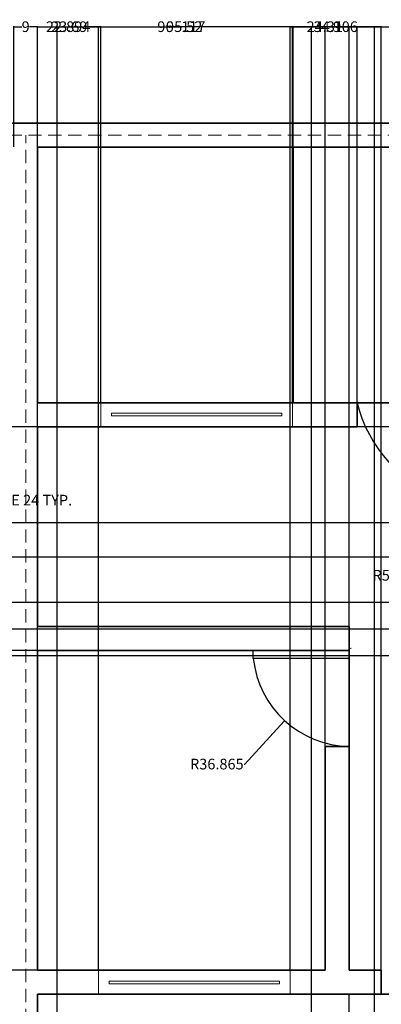
# Model space of a CAD drawing. Units: inches. Extents: x 1291 to 2095, y 532 to 1090.
# Tile 13 of 14: x 1696 to 1832, y 720 to 1090. Entities that reach past the tile are written whole.
import ezdxf

# ---------------------------------------------------------------- set-up
doc = ezdxf.new("R2010")
doc.units = ezdxf.units.IN
doc.header["$MEASUREMENT"] = 0
doc.linetypes.add('HIDDEN', pattern=[0.375, 0.25, -0.125])
for name, color, linetype, lineweight in [('A-ANNO-DIMS', 2, 'Continuous', 18), ('A-DOOR', 3, 'Continuous', 25), ('A-GLAZ', 4, 'Continuous', 18), ('A-WALL', 7, 'Continuous', 35), ('A-WALL-HIDN', 8, 'HIDDEN', 13), ('A-WALL-SITE', 7, 'Continuous', 25)]:
    doc.layers.add(name, color=color, linetype=linetype, lineweight=lineweight)
doc.styles.get("Standard").update_dxf_attribs({"font": 'arial.ttf'})
doc.dimstyles.get("Standard").update_dxf_attribs({"dimtxt": 4, "dimasz": 0.18, "dimexe": 0.18, "dimexo": 0.0625, "dimgap": 0.09, "dimtad": 0, "dimtih": 1, "dimtoh": 1, "dimdec": 0, "dimrnd": 6, "dimzin": 0, "dimdsep": 46, "dimlunit": 3, "dimtxsty": 'Standard', "dimcen": 0.09, "dimadec": 0, "dimazin": 0, "dimtfac": 1, "dimtdec": 0, "dimtofl": 0, "dimtmove": 0, "dimatfit": 3, "dimfxl": 1, "dimtolj": 1, "dimtzin": 0, "dimarcsym": 0})

# ---------------------------------------------------------------- blocks, each defined once
blk = doc.blocks.new('WIN-72IN')
for points in [[(0, 0), (0, 9), (72, 9), (72, 0)], [(4, 4), (4, 5), (68, 5), (68, 4)]]:
    blk.add_lwpolyline(points, close=True)
blk = doc.blocks.new('FRONT-COURT-DIVIDER')
for p, q in [((9.46, 23.64), (9.46, 144)), ((5, 99.92), (9.46, 99.92)), ((0, 0), (0, 94.92)), ((19.66, 85.14), (9.46, 85.14)), ((17.66, 85.14), (17.66, 23.64)), ((19.66, 85.14), (19.66, 0)), ((19.66, 23.64), (0, 23.64)), ((17.66, 21.64), (0, 21.64)), ((17.66, 21.64), (17.66, 2)), ((0, 2), (17.66, 2))]:
    blk.add_line(p, q)
blk.add_arc((5, 94.92), 5, 90, 180)
blk = doc.blocks.new('*D20')
at = {"layer": 'A-ANNO-DIMS', "color": 0, "lineweight": -2, "transparency": 16777216}
for p, q in [((1641.64, 912.72), (1641.64, 909.06)), ((1665.26, 912.72), (1665.26, 909.06)), ((1641.82, 909.24), (1665.08, 909.24)), ((1665.26, 909.24), (1665.44, 909.24))]:
    blk.add_line(p, q, dxfattribs=at)
at = {"layer": 'A-ANNO-DIMS', "color": 0, "transparency": 16777216}
for points in [[(1641.82, 909.27), (1641.82, 909.21), (1641.64, 909.24)], [(1665.08, 909.27), (1665.08, 909.21), (1665.26, 909.24)]]:
    blk.add_solid(points, dxfattribs=at)
at = {"layer": 'Defpoints', "color": 0, "transparency": 16777216}
for p in [(1641.64, 912.78), (1665.26, 912.78), (1665.26, 909.24)]:
    blk.add_point(p, dxfattribs=at)
at = {"layer": 'A-ANNO-DIMS', "color": 0, "transparency": 16777216, "insert": (1691.84, 909.24), "char_height": 4, "attachment_point": 5}
blk.add_mtext('\\A1;APPLIANCE 24 TYP.', dxfattribs=at)
blk = doc.blocks.new('*D40')
at = {"layer": 'A-ANNO-DIMS', "color": 0, "lineweight": -2, "transparency": 16777216}
for p, q in [((1694.07, 1041.84), (1694.07, 1087.16)), ((1694.25, 1086.98), (1697.17, 1086.98)), ((1702.89, 1086.98), (1699.98, 1086.98)), ((1703.07, 1041.84), (1703.07, 1087.16))]:
    blk.add_line(p, q, dxfattribs=at)
at = {"layer": 'A-ANNO-DIMS', "color": 0, "transparency": 16777216}
for points in [[(1694.25, 1087.01), (1694.25, 1086.95), (1694.07, 1086.98)], [(1702.89, 1087.01), (1702.89, 1086.95), (1703.07, 1086.98)]]:
    blk.add_solid(points, dxfattribs=at)
at = {"layer": 'Defpoints', "color": 0, "transparency": 16777216}
for p in [(1703.07, 1086.98), (1694.07, 1041.78), (1703.07, 1041.78)]:
    blk.add_point(p, dxfattribs=at)
at = {"layer": 'A-ANNO-DIMS', "color": 0, "transparency": 16777216, "insert": (1698.57, 1086.98), "char_height": 4, "attachment_point": 5}
blk.add_mtext('\\A1;9', dxfattribs=at)
blk = doc.blocks.new('*D41')
at = {"layer": 'A-ANNO-DIMS', "color": 0, "lineweight": -2, "transparency": 16777216}
for p, q in [((1703.07, 1041.84), (1703.07, 1087.16)), ((1703.25, 1086.98), (1748.12, 1086.98)), ((1798.89, 1086.98), (1754.03, 1086.98)), ((1799.07, 1041.84), (1799.07, 1087.16))]:
    blk.add_line(p, q, dxfattribs=at)
at = {"layer": 'A-ANNO-DIMS', "color": 0, "transparency": 16777216}
for points in [[(1703.25, 1087.01), (1703.25, 1086.95), (1703.07, 1086.98)], [(1798.89, 1087.01), (1798.89, 1086.95), (1799.07, 1086.98)]]:
    blk.add_solid(points, dxfattribs=at)
at = {"layer": 'Defpoints', "color": 0, "transparency": 16777216}
for p in [(1799.07, 1086.98), (1703.07, 1041.78), (1799.07, 1041.78)]:
    blk.add_point(p, dxfattribs=at)
at = {"layer": 'A-ANNO-DIMS', "color": 0, "transparency": 16777216, "insert": (1751.07, 1086.98), "char_height": 4, "attachment_point": 5}
blk.add_mtext('\\A1;96', dxfattribs=at)
blk = doc.blocks.new('*D42')
at = {"layer": 'A-ANNO-DIMS', "color": 0, "lineweight": -2, "transparency": 16777216}
for p, q in [((1799.07, 1041.84), (1799.07, 1087.16)), ((1799.25, 1086.98), (1917.53, 1086.98)), ((2044.89, 1086.98), (1926.62, 1086.98)), ((2045.07, 1041.84), (2045.07, 1087.16))]:
    blk.add_line(p, q, dxfattribs=at)
at = {"layer": 'A-ANNO-DIMS', "color": 0, "transparency": 16777216}
for points in [[(1799.25, 1087.01), (1799.25, 1086.95), (1799.07, 1086.98)], [(2044.89, 1087.01), (2044.89, 1086.95), (2045.07, 1086.98)]]:
    blk.add_solid(points, dxfattribs=at)
at = {"layer": 'Defpoints', "color": 0, "transparency": 16777216}
for p in [(2045.07, 1086.98), (1799.07, 1041.78), (2045.07, 1041.78)]:
    blk.add_point(p, dxfattribs=at)
at = {"layer": 'A-ANNO-DIMS', "color": 0, "transparency": 16777216, "insert": (1922.07, 1086.98), "char_height": 4, "attachment_point": 5}
blk.add_mtext('\\A1;246', dxfattribs=at)
blk = doc.blocks.new('*D45')
at = {"layer": 'A-ANNO-DIMS', "color": 0, "lineweight": -2, "transparency": 16777216}
for p, q in [((1829.54, 579.84), (1829.54, 1087.16)), ((1829.72, 1086.98), (1928.89, 1086.98)), ((2044.89, 1086.98), (1945.72, 1086.98)), ((2045.07, 579.84), (2045.07, 1087.16))]:
    blk.add_line(p, q, dxfattribs=at)
at = {"layer": 'A-ANNO-DIMS', "color": 0, "transparency": 16777216}
for points in [[(1829.72, 1087.01), (1829.72, 1086.95), (1829.54, 1086.98)], [(2044.89, 1087.01), (2044.89, 1086.95), (2045.07, 1086.98)]]:
    blk.add_solid(points, dxfattribs=at)
at = {"layer": 'Defpoints', "color": 0, "transparency": 16777216}
for p in [(2045.07, 1086.98), (1829.54, 579.78), (2045.07, 579.78)]:
    blk.add_point(p, dxfattribs=at)
at = {"layer": 'A-ANNO-DIMS', "color": 0, "transparency": 16777216, "insert": (1937.3, 1086.98), "char_height": 4, "attachment_point": 5}
blk.add_mtext('\\A1;215.54', dxfattribs=at)
blk = doc.blocks.new('*D47')
at = {"layer": 'A-ANNO-DIMS', "color": 0, "lineweight": -2, "transparency": 16777216}
for p, q in [((1710.36, 579.84), (1710.36, 1087.16)), ((1710.54, 1086.98), (1751.3, 1086.98)), ((1805.7, 1086.98), (1764.94, 1086.98)), ((1805.88, 579.84), (1805.88, 1087.16))]:
    blk.add_line(p, q, dxfattribs=at)
at = {"layer": 'A-ANNO-DIMS', "color": 0, "transparency": 16777216}
for points in [[(1710.54, 1087.01), (1710.54, 1086.95), (1710.36, 1086.98)], [(1805.7, 1087.01), (1805.7, 1086.95), (1805.88, 1086.98)]]:
    blk.add_solid(points, dxfattribs=at)
at = {"layer": 'Defpoints', "color": 0, "transparency": 16777216}
for p in [(1805.88, 1086.98), (1710.36, 579.78), (1805.88, 579.78)]:
    blk.add_point(p, dxfattribs=at)
at = {"layer": 'A-ANNO-DIMS', "color": 0, "transparency": 16777216, "insert": (1758.12, 1086.98), "char_height": 4, "attachment_point": 5}
blk.add_mtext('\\A1;95.52', dxfattribs=at)
blk = doc.blocks.new('*D50')
at = {"layer": 'A-ANNO-DIMS', "color": 0, "lineweight": -2, "transparency": 16777216}
for p, q in [((1703.07, 861.84), (1703.07, 1087.16)), ((1703.25, 1086.98), (1757.25, 1086.98)), ((1819.89, 1086.98), (1765.89, 1086.98)), ((1820.07, 861.84), (1820.07, 1087.16))]:
    blk.add_line(p, q, dxfattribs=at)
at = {"layer": 'A-ANNO-DIMS', "color": 0, "transparency": 16777216}
for points in [[(1703.25, 1087.01), (1703.25, 1086.95), (1703.07, 1086.98)], [(1819.89, 1087.01), (1819.89, 1086.95), (1820.07, 1086.98)]]:
    blk.add_solid(points, dxfattribs=at)
at = {"layer": 'Defpoints', "color": 0, "transparency": 16777216}
for p in [(1820.07, 1086.98), (1703.07, 861.78), (1820.07, 861.78)]:
    blk.add_point(p, dxfattribs=at)
at = {"layer": 'A-ANNO-DIMS', "color": 0, "transparency": 16777216, "insert": (1761.57, 1086.98), "char_height": 4, "attachment_point": 5}
blk.add_mtext('\\A1;117', dxfattribs=at)
blk = doc.blocks.new('*D51')
at = {"layer": 'A-ANNO-DIMS', "color": 0, "lineweight": -2, "transparency": 16777216}
for p, q in [((1820.01, 852.78), (1297.69, 852.78)), ((1297.87, 852.6), (1297.87, 794.91)), ((1297.87, 732.96), (1297.87, 790.65)), ((1811.01, 732.78), (1297.69, 732.78))]:
    blk.add_line(p, q, dxfattribs=at)
at = {"layer": 'A-ANNO-DIMS', "color": 0, "transparency": 16777216}
for points in [[(1297.84, 852.6), (1297.9, 852.6), (1297.87, 852.78)], [(1297.84, 732.96), (1297.9, 732.96), (1297.87, 732.78)]]:
    blk.add_solid(points, dxfattribs=at)
at = {"layer": 'Defpoints', "color": 0, "transparency": 16777216}
for p in [(1297.87, 852.78), (1820.07, 852.78), (1811.07, 732.78)]:
    blk.add_point(p, dxfattribs=at)
at = {"layer": 'A-ANNO-DIMS', "color": 0, "transparency": 16777216, "insert": (1297.87, 792.78), "char_height": 4, "attachment_point": 5}
blk.add_mtext('\\A1;120', dxfattribs=at)
blk = doc.blocks.new('*D52')
at = {"layer": 'A-ANNO-DIMS', "color": 0, "lineweight": -2, "transparency": 16777216}
for p, q in [((1811.07, 816.84), (1811.07, 1087.16)), ((1811.25, 1086.98), (1814.17, 1086.98)), ((1819.89, 1086.98), (1816.98, 1086.98)), ((1820.07, 816.84), (1820.07, 1087.16))]:
    blk.add_line(p, q, dxfattribs=at)
at = {"layer": 'A-ANNO-DIMS', "color": 0, "transparency": 16777216}
for points in [[(1811.25, 1087.01), (1811.25, 1086.95), (1811.07, 1086.98)], [(1819.89, 1087.01), (1819.89, 1086.95), (1820.07, 1086.98)]]:
    blk.add_solid(points, dxfattribs=at)
at = {"layer": 'Defpoints', "color": 0, "transparency": 16777216}
for p in [(1820.07, 1086.98), (1811.07, 816.78), (1820.07, 816.78)]:
    blk.add_point(p, dxfattribs=at)
at = {"layer": 'A-ANNO-DIMS', "color": 0, "transparency": 16777216, "insert": (1815.57, 1086.98), "char_height": 4, "attachment_point": 5}
blk.add_mtext('\\A1;9', dxfattribs=at)
blk = doc.blocks.new('*D56')
at = {"layer": 'A-ANNO-DIMS', "color": 0, "lineweight": -2, "transparency": 16777216}
for p, q in [((1868.01, 936.78), (1297.69, 936.78)), ((1297.87, 936.6), (1297.87, 914.41)), ((1297.87, 887.96), (1297.87, 910.15)), ((1868.01, 887.78), (1297.69, 887.78))]:
    blk.add_line(p, q, dxfattribs=at)
at = {"layer": 'A-ANNO-DIMS', "color": 0, "transparency": 16777216}
for points in [[(1297.84, 936.6), (1297.9, 936.6), (1297.87, 936.78)], [(1297.84, 887.96), (1297.9, 887.96), (1297.87, 887.78)]]:
    blk.add_solid(points, dxfattribs=at)
at = {"layer": 'Defpoints', "color": 0, "transparency": 16777216}
for p in [(1297.87, 936.78), (1868.07, 936.78), (1868.07, 887.78)]:
    blk.add_point(p, dxfattribs=at)
at = {"layer": 'A-ANNO-DIMS', "color": 0, "transparency": 16777216, "insert": (1297.87, 912.28), "char_height": 4, "attachment_point": 5}
blk.add_mtext('\\A1;49', dxfattribs=at)
blk = doc.blocks.new('*D57')
at = {"layer": 'A-ANNO-DIMS', "color": 0, "lineweight": -2, "transparency": 16777216}
for p, q in [((1973.01, 900.78), (1297.69, 900.78)), ((1297.87, 900.6), (1297.87, 896.41)), ((1297.87, 887.96), (1297.87, 892.15)), ((1973.01, 887.78), (1297.69, 887.78))]:
    blk.add_line(p, q, dxfattribs=at)
at = {"layer": 'A-ANNO-DIMS', "color": 0, "transparency": 16777216}
for points in [[(1297.84, 900.6), (1297.9, 900.6), (1297.87, 900.78)], [(1297.84, 887.96), (1297.9, 887.96), (1297.87, 887.78)]]:
    blk.add_solid(points, dxfattribs=at)
at = {"layer": 'Defpoints', "color": 0, "transparency": 16777216}
for p in [(1297.87, 900.78), (1973.07, 900.78), (1973.07, 887.78)]:
    blk.add_point(p, dxfattribs=at)
at = {"layer": 'A-ANNO-DIMS', "color": 0, "transparency": 16777216, "insert": (1297.87, 894.28), "char_height": 4, "attachment_point": 5}
blk.add_mtext('\\A1;13', dxfattribs=at)
blk = doc.blocks.new('*D59')
at = {"layer": 'A-ANNO-DIMS', "color": 0, "lineweight": -2, "transparency": 16777216}
for p, q in [((2009.01, 900.78), (1297.69, 900.78)), ((1297.87, 900.6), (1297.87, 877.91)), ((1297.87, 850.96), (1297.87, 873.65)), ((2009.01, 850.78), (1297.69, 850.78))]:
    blk.add_line(p, q, dxfattribs=at)
at = {"layer": 'A-ANNO-DIMS', "color": 0, "transparency": 16777216}
for points in [[(1297.84, 900.6), (1297.9, 900.6), (1297.87, 900.78)], [(1297.84, 850.96), (1297.9, 850.96), (1297.87, 850.78)]]:
    blk.add_solid(points, dxfattribs=at)
at = {"layer": 'Defpoints', "color": 0, "transparency": 16777216}
for p in [(1297.87, 900.78), (2009.07, 900.78), (2009.07, 850.78)]:
    blk.add_point(p, dxfattribs=at)
at = {"layer": 'A-ANNO-DIMS', "color": 0, "transparency": 16777216, "insert": (1297.87, 875.78), "char_height": 4, "attachment_point": 5}
blk.add_mtext('\\A1;50', dxfattribs=at)
blk = doc.blocks.new('*D60')
at = {"layer": 'A-ANNO-DIMS', "color": 0, "lineweight": -2, "transparency": 16777216}
for p, q in [((2045.01, 870.78), (1297.69, 870.78)), ((1297.87, 870.6), (1297.87, 867.91)), ((1297.87, 860.96), (1297.87, 863.65)), ((2045.01, 860.78), (1297.69, 860.78))]:
    blk.add_line(p, q, dxfattribs=at)
at = {"layer": 'A-ANNO-DIMS', "color": 0, "transparency": 16777216}
for points in [[(1297.84, 870.6), (1297.9, 870.6), (1297.87, 870.78)], [(1297.84, 860.96), (1297.9, 860.96), (1297.87, 860.78)]]:
    blk.add_solid(points, dxfattribs=at)
at = {"layer": 'Defpoints', "color": 0, "transparency": 16777216}
for p in [(1297.87, 870.78), (2045.07, 870.78), (2045.07, 860.78)]:
    blk.add_point(p, dxfattribs=at)
at = {"layer": 'A-ANNO-DIMS', "color": 0, "transparency": 16777216, "insert": (1297.87, 865.78), "char_height": 4, "attachment_point": 5}
blk.add_mtext('\\A1;10', dxfattribs=at)
blk = doc.blocks.new('*D65')
at = {"layer": 'A-ANNO-DIMS', "color": 0, "lineweight": -2, "transparency": 16777216}
for p, q in [((1703.07, 732.84), (1703.07, 1087.16)), ((1703.25, 1086.98), (1706.1, 1086.98)), ((1725.79, 1086.98), (1722.94, 1086.98)), ((1725.97, 732.69), (1725.97, 1087.16))]:
    blk.add_line(p, q, dxfattribs=at)
at = {"layer": 'A-ANNO-DIMS', "color": 0, "transparency": 16777216}
for points in [[(1703.25, 1087.01), (1703.25, 1086.95), (1703.07, 1086.98)], [(1725.79, 1087.01), (1725.79, 1086.95), (1725.97, 1086.98)]]:
    blk.add_solid(points, dxfattribs=at)
at = {"layer": 'Defpoints', "color": 0, "transparency": 16777216}
for p in [(1725.97, 1086.98), (1703.07, 732.78), (1725.97, 732.63)]:
    blk.add_point(p, dxfattribs=at)
at = {"layer": 'A-ANNO-DIMS', "color": 0, "transparency": 16777216, "insert": (1714.52, 1086.98), "char_height": 4, "attachment_point": 5}
blk.add_mtext('\\A1;22.894', dxfattribs=at)
blk = doc.blocks.new('*D66')
at = {"layer": 'A-ANNO-DIMS', "color": 0, "lineweight": -2, "transparency": 16777216}
for p, q in [((1797.97, 732.69), (1797.97, 1087.16)), ((1798.15, 1086.98), (1806.63, 1086.98)), ((1831.89, 1086.98), (1823.41, 1086.98)), ((1832.07, 732.84), (1832.07, 1087.16))]:
    blk.add_line(p, q, dxfattribs=at)
at = {"layer": 'A-ANNO-DIMS', "color": 0, "transparency": 16777216}
for points in [[(1798.15, 1087.01), (1798.15, 1086.95), (1797.97, 1086.98)], [(1831.89, 1087.01), (1831.89, 1086.95), (1832.07, 1086.98)]]:
    blk.add_solid(points, dxfattribs=at)
at = {"layer": 'Defpoints', "color": 0, "transparency": 16777216}
for p in [(1832.07, 1086.98), (1797.97, 732.63), (1832.07, 732.78)]:
    blk.add_point(p, dxfattribs=at)
at = {"layer": 'A-ANNO-DIMS', "color": 0, "transparency": 16777216, "insert": (1815.02, 1086.98), "char_height": 4, "attachment_point": 5}
blk.add_mtext('\\A1;34.106', dxfattribs=at)
blk = doc.blocks.new('*D67')
at = {"layer": 'A-ANNO-DIMS', "color": 0, "lineweight": -2, "transparency": 16777216}
for p, q in [((1832.07, 723.84), (1832.07, 1087.16)), ((1832.25, 1086.98), (1847.12, 1086.98)), ((1867.89, 1086.98), (1853.03, 1086.98)), ((1868.07, 723.84), (1868.07, 1087.16))]:
    blk.add_line(p, q, dxfattribs=at)
at = {"layer": 'A-ANNO-DIMS', "color": 0, "transparency": 16777216}
for points in [[(1832.25, 1087.01), (1832.25, 1086.95), (1832.07, 1086.98)], [(1867.89, 1087.01), (1867.89, 1086.95), (1868.07, 1086.98)]]:
    blk.add_solid(points, dxfattribs=at)
at = {"layer": 'Defpoints', "color": 0, "transparency": 16777216}
for p in [(1868.07, 1086.98), (1832.07, 723.78), (1868.07, 723.78)]:
    blk.add_point(p, dxfattribs=at)
at = {"layer": 'A-ANNO-DIMS', "color": 0, "transparency": 16777216, "insert": (1850.07, 1086.98), "char_height": 4, "attachment_point": 5}
blk.add_mtext('\\A1;36', dxfattribs=at)
blk = doc.blocks.new('*D73')
at = {"layer": 'A-ANNO-DIMS', "color": 0, "lineweight": -2, "transparency": 16777216}
for p, q in [((1703.07, 945.84), (1703.07, 1087.16)), ((1703.25, 1086.98), (1708.04, 1086.98)), ((1726.58, 1086.98), (1721.79, 1086.98)), ((1726.76, 946.01), (1726.76, 1087.16))]:
    blk.add_line(p, q, dxfattribs=at)
at = {"layer": 'A-ANNO-DIMS', "color": 0, "transparency": 16777216}
for points in [[(1703.25, 1087.01), (1703.25, 1086.95), (1703.07, 1086.98)], [(1726.58, 1087.01), (1726.58, 1086.95), (1726.76, 1086.98)]]:
    blk.add_solid(points, dxfattribs=at)
at = {"layer": 'Defpoints', "color": 0, "transparency": 16777216}
for p in [(1726.76, 1086.98), (1703.07, 945.78), (1726.76, 945.95)]:
    blk.add_point(p, dxfattribs=at)
at = {"layer": 'A-ANNO-DIMS', "color": 0, "transparency": 16777216, "insert": (1714.92, 1086.98), "char_height": 4, "attachment_point": 5}
blk.add_mtext('\\A1;23.69', dxfattribs=at)
blk = doc.blocks.new('*D74')
at = {"layer": 'A-ANNO-DIMS', "color": 0, "lineweight": -2, "transparency": 16777216}
for p, q in [((1798.76, 946.01), (1798.76, 1087.16)), ((1798.94, 1086.98), (1804.43, 1086.98)), ((1822.89, 1086.98), (1817.4, 1086.98)), ((1823.07, 945.84), (1823.07, 1087.16))]:
    blk.add_line(p, q, dxfattribs=at)
at = {"layer": 'A-ANNO-DIMS', "color": 0, "transparency": 16777216}
for points in [[(1798.94, 1087.01), (1798.94, 1086.95), (1798.76, 1086.98)], [(1822.89, 1087.01), (1822.89, 1086.95), (1823.07, 1086.98)]]:
    blk.add_solid(points, dxfattribs=at)
at = {"layer": 'Defpoints', "color": 0, "transparency": 16777216}
for p in [(1823.07, 1086.98), (1798.76, 945.95), (1823.07, 945.78)]:
    blk.add_point(p, dxfattribs=at)
at = {"layer": 'A-ANNO-DIMS', "color": 0, "transparency": 16777216, "insert": (1810.92, 1086.98), "char_height": 4, "attachment_point": 5}
blk.add_mtext('\\A1;24.31', dxfattribs=at)
blk = doc.blocks.new('*D75')
at = {"layer": 'A-ANNO-DIMS', "color": 0, "lineweight": -2, "transparency": 16777216}
for p, q in [((1823.07, 945.84), (1823.07, 1087.16)), ((1823.25, 1086.98), (1838.12, 1086.98)), ((1858.89, 1086.98), (1844.03, 1086.98)), ((1859.07, 945.84), (1859.07, 1087.16))]:
    blk.add_line(p, q, dxfattribs=at)
at = {"layer": 'A-ANNO-DIMS', "color": 0, "transparency": 16777216}
for points in [[(1823.25, 1087.01), (1823.25, 1086.95), (1823.07, 1086.98)], [(1858.89, 1087.01), (1858.89, 1086.95), (1859.07, 1086.98)]]:
    blk.add_solid(points, dxfattribs=at)
at = {"layer": 'Defpoints', "color": 0, "transparency": 16777216}
for p in [(1859.07, 1086.98), (1823.07, 945.78), (1859.07, 945.78)]:
    blk.add_point(p, dxfattribs=at)
at = {"layer": 'A-ANNO-DIMS', "color": 0, "transparency": 16777216, "insert": (1841.07, 1086.98), "char_height": 4, "attachment_point": 5}
blk.add_mtext('\\A1;36', dxfattribs=at)
blk = doc.blocks.new('*D86')
at = {"layer": 'A-ANNO-DIMS', "color": 0, "lineweight": -2, "transparency": 16777216}
for p, q in [((1820.65, 853.64), (1820.83, 853.64)), ((1820.74, 853.55), (1820.74, 853.73)), ((1780.88, 810.16), (1795.7, 826.33)), ((1780.7, 810.16), (1780.88, 810.16))]:
    blk.add_line(p, q, dxfattribs=at)
at = {"layer": 'A-ANNO-DIMS', "color": 0, "transparency": 16777216}
blk.add_solid([(1795.68, 826.35), (1795.73, 826.31), (1795.83, 826.46)], dxfattribs=at)
at = {"layer": 'Defpoints', "color": 0, "transparency": 16777216}
for p in [(1820.74, 853.64), (1795.83, 826.46)]:
    blk.add_point(p, dxfattribs=at)
at = {"layer": 'A-ANNO-DIMS', "color": 0, "transparency": 16777216, "insert": (1770.38, 810.16), "char_height": 4, "attachment_point": 5}
blk.add_mtext('\\A1;R36.865', dxfattribs=at)
blk = doc.blocks.new('*D91')
at = {"layer": 'A-ANNO-DIMS', "color": 0, "lineweight": -2, "transparency": 16777216}
for p, q in [((1872.33, 957.89), (1872.51, 957.89)), ((1872.42, 957.8), (1872.42, 957.98)), ((1845.96, 881.02), (1855.82, 909.68)), ((1845.78, 881.02), (1845.96, 881.02))]:
    blk.add_line(p, q, dxfattribs=at)
at = {"layer": 'A-ANNO-DIMS', "color": 0, "transparency": 16777216}
blk.add_solid([(1855.79, 909.69), (1855.85, 909.67), (1855.88, 909.85)], dxfattribs=at)
at = {"layer": 'Defpoints', "color": 0, "transparency": 16777216}
for p in [(1872.42, 957.89), (1855.88, 909.85)]:
    blk.add_point(p, dxfattribs=at)
at = {"layer": 'A-ANNO-DIMS', "color": 0, "transparency": 16777216, "insert": (1837.41, 881.02), "char_height": 4, "attachment_point": 5}
blk.add_mtext('\\A1;R50.81', dxfattribs=at)

msp = doc.modelspace()

# ---------------------------------------------------------------- linework, layer by layer
at = {"layer": 'A-DOOR'}
msp.add_lwpolyline([(1820.0735, 852.7804), (1820.0735, 849.7804), (1784.0735, 849.7804), (1784.0735, 852.7804)], close=True, dxfattribs=at)
for centre, radius, start, end in [((1872.4221, 957.8916), 50.813, 193.789075, 251.231819), ((1820.7362, 853.6397), 36.8653, 186.009135, 268.969971)]:
    msp.add_arc(centre, radius, start, end, dxfattribs=at)
at = {"layer": 'A-WALL'}
for p, q in [((2054.0735, 1050.7804), (1334.0735, 1050.7804)), ((2045.0735, 1041.7804), (1703.0735, 1041.7804)), ((1703.0735, 945.7804), (1703.0735, 1041.7804)), ((1799.0735, 945.7804), (1799.0735, 1041.7804)), ((1856.0735, 945.7804), (1703.0735, 945.7804)), ((1823.0735, 936.7804), (1823.0735, 945.7804)), ((1703.0735, 861.7804), (1703.0735, 936.7804)), ((1823.0735, 936.7804), (1703.0735, 936.7804)), ((1820.0735, 861.7804), (1703.0735, 861.7804)), ((1820.0735, 852.7804), (1820.0735, 861.7804)), ((1820.0735, 852.7804), (1703.0735, 852.7804)), ((1703.0735, 732.7804), (1703.0735, 852.7804)), ((1820.0735, 732.7804), (1820.0735, 849.7804)), ((1811.0735, 732.7804), (1811.0735, 816.7804)), ((1820.0735, 816.7804), (1811.0735, 816.7804)), ((1703.0735, 732.7804), (1811.0735, 732.7804)), ((1820.0735, 732.7804), (1832.0735, 732.7804)), ((1832.0735, 723.7804), (1832.0735, 732.7804)), ((1703.0735, 579.7804), (1703.0735, 723.7804)), ((1703.0735, 723.7804), (1868.0735, 723.7804))]:
    msp.add_line(p, q, dxfattribs=at)
at = {"layer": 'A-WALL-HIDN', "ltscale": 20}
for p, q in [((2049.5735, 1046.2804), (1338.5735, 1046.2804)), ((1698.5735, 570.7804), (1698.5735, 1046.2804))]:
    msp.add_line(p, q, dxfattribs=at)

# ---------------------------------------------------------------- block references
at = {"layer": 'A-GLAZ'}
for p in [(1726.7622, 936.9457), (1725.9681, 723.6289)]:
    msp.add_blockref('WIN-72IN', p, dxfattribs=at)
at = {"layer": 'A-WALL-SITE', "extrusion": (0, 0, -1), "zscale": -1}
msp.add_blockref('FRONT-COURT-DIVIDER', (-1829.5361, 579.78), dxfattribs=at)

# ---------------------------------------------------------------- dimensions: what is measured, and where the dimension line sits
at = {"layer": 'A-ANNO-DIMS'}
for base, p1, p2, override, picture, middle in [((1703.0735, 1086.9804), (1694.0735, 1041.7804), (1703.0735, 1041.7804), {"dimdec": 0, "dimlfac": 1, "dimrnd": 0, "dimzin": 0, "dimdsep": 46, "dimlunit": 2}, '*D40', (1698.5735, 1086.9804)), ((1799.0735, 1086.9804), (1703.0735, 1041.7804), (1799.0735, 1041.7804), {"dimdec": 0, "dimlfac": 1, "dimrnd": 0, "dimzin": 0, "dimdsep": 46, "dimlunit": 2}, '*D41', (1751.0735, 1086.9804)), ((1820.0735, 1086.9804), (1703.0735, 861.7804), (1820.0735, 861.7804), {"dimdec": 0, "dimlfac": 1, "dimrnd": 0, "dimzin": 0, "dimdsep": 46, "dimlunit": 2}, '*D50', (1761.5735, 1086.9804)), ((1725.9677, 1086.9804), (1703.0735, 732.7804), (1725.9677, 732.6285), {"dimdec": 3, "dimlfac": 1, "dimrnd": 0, "dimzin": 0, "dimdsep": 46, "dimlunit": 2}, '*D65', (1714.5206, 1086.9804)), ((1726.7618, 1086.9804), (1703.0735, 945.7804), (1726.7618, 945.9453), {"dimdec": 2, "dimlfac": 1, "dimrnd": 0, "dimzin": 0, "dimdsep": 46, "dimlunit": 2}, '*D73', (1714.9177, 1086.9804)), ((1805.8774, 1086.9804), (1710.3593, 579.7804), (1805.8774, 579.7804), {"dimdec": 2, "dimlfac": 1, "dimrnd": 0, "dimzin": 0, "dimdsep": 46, "dimlunit": 2}, '*D47', (1758.1183, 1086.9804)), ((1832.0735, 1086.9804), (1797.9677, 732.6285), (1832.0735, 732.7804), {"dimdec": 3, "dimlfac": 1, "dimrnd": 0, "dimzin": 0, "dimdsep": 46, "dimlunit": 2}, '*D66', (1815.0206, 1086.9804)), ((1823.0735, 1086.9804), (1798.7618, 945.9453), (1823.0735, 945.7804), {"dimdec": 2, "dimlfac": 1, "dimrnd": 0, "dimzin": 0, "dimdsep": 46, "dimlunit": 2}, '*D74', (1810.9177, 1086.9804)), ((2045.0735, 1086.9804), (1799.0735, 1041.7804), (2045.0735, 1041.7804), {"dimdec": 0, "dimlfac": 1, "dimrnd": 0, "dimzin": 0, "dimdsep": 46, "dimlunit": 2}, '*D42', (1922.0735, 1086.9804)), ((1820.0735, 1086.9804), (1811.0735, 816.7804), (1820.0735, 816.7804), {"dimdec": 0, "dimlfac": 1, "dimrnd": 0, "dimzin": 0, "dimdsep": 46, "dimlunit": 2}, '*D52', (1815.5735, 1086.9804)), ((1859.0735, 1086.9804), (1823.0735, 945.7804), (1859.0735, 945.7804), {"dimdec": 0, "dimlfac": 1, "dimrnd": 0, "dimzin": 0, "dimdsep": 46, "dimlunit": 2}, '*D75', (1841.0735, 1086.9804)), ((2045.0735, 1086.9804), (1829.5364, 579.7804), (2045.0735, 579.7804), {"dimdec": 2, "dimlfac": 1, "dimrnd": 0, "dimzin": 0, "dimdsep": 46, "dimlunit": 2}, '*D45', (1937.3049, 1086.9804)), ((1868.0735, 1086.9804), (1832.0735, 723.7804), (1868.0735, 723.7804), {"dimdec": 0, "dimlfac": 1, "dimrnd": 0, "dimzin": 0, "dimdsep": 46, "dimlunit": 2}, '*D67', (1850.0735, 1086.9804))]:
    dim = msp.add_linear_dim(base=base, p1=p1, p2=p2, dimstyle='Standard', override=override, dxfattribs=at)
    dim.commit()
    dim.dimension.update_dxf_attribs({"geometry": picture, "text_midpoint": middle})
for center, mpoint, override, picture, middle in [((1872.4221, 957.8916), (1855.8814, 909.8461), {"dimdec": 2, "dimlfac": 1, "dimrnd": 0, "dimzin": 0, "dimdsep": 46, "dimlunit": 2}, '*D91', (1837.4101, 881.0188)), ((1820.7362, 853.6397), (1795.8254, 826.4644), {"dimdec": 3, "dimlfac": 1, "dimrnd": 0, "dimzin": 0, "dimdsep": 46, "dimlunit": 2}, '*D86', (1770.3769, 810.1592))]:
    dim = msp.add_radius_dim(center=center, mpoint=mpoint, dimstyle='Standard', override=override, dxfattribs=at)
    dim.commit()
    dim.dimension.update_dxf_attribs({"geometry": picture, "text_midpoint": middle, "dimtype": 164})
for base, p1, p2, picture, middle in [((1297.8735, 936.7804), (1868.0735, 887.7804), (1868.0735, 936.7804), '*D56', (1297.8735, 912.2804)), ((1297.8735, 900.7804), (1973.0735, 887.7804), (1973.0735, 900.7804), '*D57', (1297.8735, 894.2804)), ((1297.8735, 900.7804), (2009.0735, 850.7804), (2009.0735, 900.7804), '*D59', (1297.8735, 875.7804)), ((1297.8735, 870.7804), (2045.0735, 860.7804), (2045.0735, 870.7804), '*D60', (1297.8735, 865.7804)), ((1297.8735, 852.7804), (1811.0735, 732.7804), (1820.0735, 852.7804), '*D51', (1297.8735, 792.7804))]:
    dim = msp.add_linear_dim(base=base, p1=p1, p2=p2, angle=90, dimstyle='Standard', override={"dimdec": 0, "dimlfac": 1, "dimrnd": 0, "dimzin": 0, "dimdsep": 46, "dimlunit": 2}, dxfattribs=at)
    dim.commit()
    dim.dimension.update_dxf_attribs({"geometry": picture, "text_midpoint": middle})
dim = msp.add_linear_dim(base=(1665.2638, 909.2371), p1=(1641.6418, 912.7804), p2=(1665.2638, 912.7804), text='APPLIANCE <> TYP.', dimstyle='Standard', override={"dimdec": 0, "dimlfac": 1, "dimrnd": 0, "dimzin": 0, "dimdsep": 46, "dimlunit": 2}, dxfattribs=at)
dim.commit()
dim.dimension.update_dxf_attribs({"geometry": '*D20', "text_midpoint": (1691.8449, 909.2371)})

doc.saveas('drawing.dxf')
